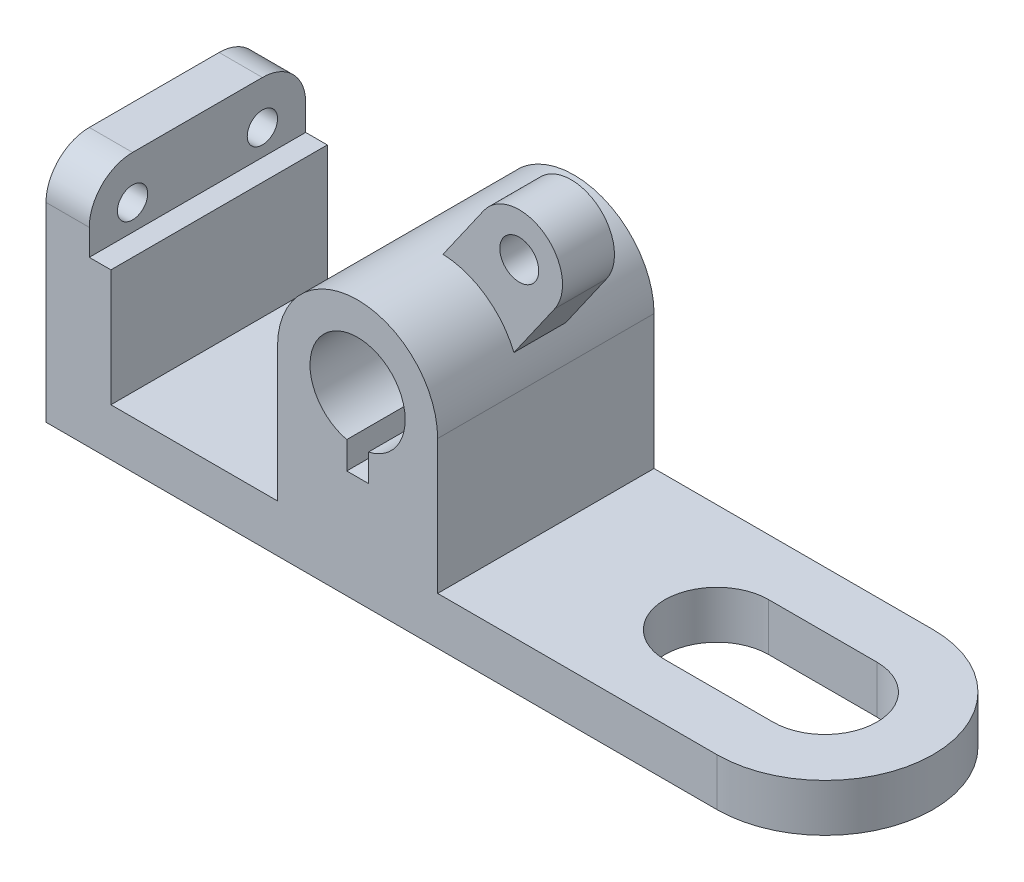
ISO-10303-21;
HEADER;
FILE_DESCRIPTION(('STEP AP214'),'2;1');
FILE_NAME('part.step','',(''),(''),'','','');
FILE_SCHEMA(('AUTOMOTIVE_DESIGN { 1 0 10303 214 1 1 1 1 }'));
ENDSEC;
DATA;
#1=APPLICATION_CONTEXT('core data for automotive mechanical design processes');
#2=APPLICATION_PROTOCOL_DEFINITION('international standard','automotive_design',2000,#1);
#3=PRODUCT_CONTEXT('',#1,'mechanical');
#4=PRODUCT('Part','Part','',(#3));
#5=PRODUCT_RELATED_PRODUCT_CATEGORY('part','',(#4));
#6=PRODUCT_DEFINITION_FORMATION('','',#4);
#7=PRODUCT_DEFINITION_CONTEXT('part definition',#1,'design');
#8=PRODUCT_DEFINITION('design','',#6,#7);
#9=PRODUCT_DEFINITION_SHAPE('','',#8);
#10=(LENGTH_UNIT() NAMED_UNIT(*) SI_UNIT(.MILLI.,.METRE.));
#11=(NAMED_UNIT(*) PLANE_ANGLE_UNIT() SI_UNIT($,.RADIAN.));
#12=(NAMED_UNIT(*) SI_UNIT($,.STERADIAN.) SOLID_ANGLE_UNIT());
#13=UNCERTAINTY_MEASURE_WITH_UNIT(LENGTH_MEASURE(1.E-05),#10,'distance_accuracy_value','');
#14=(GEOMETRIC_REPRESENTATION_CONTEXT(3) GLOBAL_UNCERTAINTY_ASSIGNED_CONTEXT((#13)) GLOBAL_UNIT_ASSIGNED_CONTEXT((#10,
#11,#12)) REPRESENTATION_CONTEXT('',''));
#15=CARTESIAN_POINT('',(0.,0.,0.));
#16=DIRECTION('',(0.,0.,1.));
#17=DIRECTION('',(1.,0.,0.));
#18=AXIS2_PLACEMENT_3D('',#15,#16,#17);
#19=CARTESIAN_POINT('',(0.,38.,0.));
#20=DIRECTION('',(0.,1.,0.));
#21=DIRECTION('',(0.,0.,1.));
#22=AXIS2_PLACEMENT_3D('',#19,#20,#21);
#23=PLANE('',#22);
#24=DIRECTION('',(-1.,0.,0.));
#25=VECTOR('',#24,1.);
#26=CARTESIAN_POINT('',(-62.5,38.,-25.));
#27=LINE('',#26,#25);
#28=CARTESIAN_POINT('',(-62.5,38.,-25.));
#29=VERTEX_POINT('',#28);
#30=CARTESIAN_POINT('',(-67.5,38.,-25.));
#31=VERTEX_POINT('',#30);
#32=EDGE_CURVE('E242',#29,#31,#27,.T.);
#33=ORIENTED_EDGE('',*,*,#32,.T.);
#34=DIRECTION('',(0.,0.,-1.));
#35=VECTOR('',#34,1.);
#36=CARTESIAN_POINT('',(-67.5,38.,25.));
#37=LINE('',#36,#35);
#38=CARTESIAN_POINT('',(-67.5,38.,25.));
#39=VERTEX_POINT('',#38);
#40=EDGE_CURVE('E221',#39,#31,#37,.T.);
#41=ORIENTED_EDGE('',*,*,#40,.F.);
#42=DIRECTION('',(1.,0.,0.));
#43=VECTOR('',#42,1.);
#44=CARTESIAN_POINT('',(-77.5,38.,25.));
#45=LINE('',#44,#43);
#46=CARTESIAN_POINT('',(-62.5,38.,25.));
#47=VERTEX_POINT('',#46);
#48=EDGE_CURVE('E218',#39,#47,#45,.T.);
#49=ORIENTED_EDGE('',*,*,#48,.T.);
#50=DIRECTION('',(0.,0.,-1.));
#51=VECTOR('',#50,1.);
#52=CARTESIAN_POINT('',(-62.5,38.,25.));
#53=LINE('',#52,#51);
#54=EDGE_CURVE('E225',#47,#29,#53,.T.);
#55=ORIENTED_EDGE('',*,*,#54,.T.);
#56=EDGE_LOOP('',(#33,#41,#49,#55));
#57=FACE_BOUND('',#56,.T.);
#58=ADVANCED_FACE('F44',(#57),#23,.T.);
#59=CARTESIAN_POINT('',(77.5,11.,0.));
#60=DIRECTION('',(0.,1.,0.));
#61=DIRECTION('',(0.,0.,1.));
#62=AXIS2_PLACEMENT_3D('',#59,#60,#61);
#63=PLANE('',#62);
#64=DIRECTION('',(-1.,0.,0.));
#65=VECTOR('',#64,1.);
#66=CARTESIAN_POINT('',(-77.5,11.,-25.));
#67=LINE('',#66,#65);
#68=CARTESIAN_POINT('',(-24.,11.,-25.));
#69=VERTEX_POINT('',#68);
#70=CARTESIAN_POINT('',(-62.5,11.,-25.));
#71=VERTEX_POINT('',#70);
#72=EDGE_CURVE('E366',#69,#71,#67,.T.);
#73=ORIENTED_EDGE('',*,*,#72,.T.);
#74=DIRECTION('',(0.,0.,-1.));
#75=VECTOR('',#74,1.);
#76=CARTESIAN_POINT('',(-62.5,11.,25.));
#77=LINE('',#76,#75);
#78=CARTESIAN_POINT('',(-62.5,11.,25.));
#79=VERTEX_POINT('',#78);
#80=EDGE_CURVE('E226',#79,#71,#77,.T.);
#81=ORIENTED_EDGE('',*,*,#80,.F.);
#82=DIRECTION('',(1.,0.,0.));
#83=VECTOR('',#82,1.);
#84=CARTESIAN_POINT('',(77.5,11.,25.));
#85=LINE('',#84,#83);
#86=CARTESIAN_POINT('',(-24.,11.,25.));
#87=VERTEX_POINT('',#86);
#88=EDGE_CURVE('E232',#79,#87,#85,.T.);
#89=ORIENTED_EDGE('',*,*,#88,.T.);
#90=DIRECTION('',(0.,0.,1.));
#91=VECTOR('',#90,1.);
#92=CARTESIAN_POINT('',(-24.,11.,-25.));
#93=LINE('',#92,#91);
#94=EDGE_CURVE('E339',#69,#87,#93,.T.);
#95=ORIENTED_EDGE('',*,*,#94,.F.);
#96=EDGE_LOOP('',(#73,#81,#89,#95));
#97=FACE_BOUND('',#96,.T.);
#98=ADVANCED_FACE('F477',(#97),#63,.T.);
#99=CARTESIAN_POINT('',(52.5,11.,0.));
#100=DIRECTION('',(0.,1.,0.));
#101=DIRECTION('',(0.,0.,1.));
#102=AXIS2_PLACEMENT_3D('',#99,#100,#101);
#103=CIRCLE('',#102,12.);
#104=CARTESIAN_POINT('',(52.5,11.,-12.));
#105=VERTEX_POINT('',#104);
#106=CARTESIAN_POINT('',(52.5,11.,12.));
#107=VERTEX_POINT('',#106);
#108=EDGE_CURVE('E331',#105,#107,#103,.T.);
#109=ORIENTED_EDGE('',*,*,#108,.F.);
#110=DIRECTION('',(-1.,0.,0.));
#111=VECTOR('',#110,1.);
#112=CARTESIAN_POINT('',(52.5,11.,-12.));
#113=LINE('',#112,#111);
#114=CARTESIAN_POINT('',(77.5,11.,-12.));
#115=VERTEX_POINT('',#114);
#116=EDGE_CURVE('E349',#115,#105,#113,.T.);
#117=ORIENTED_EDGE('',*,*,#116,.F.);
#118=CARTESIAN_POINT('',(77.5,11.,0.));
#119=DIRECTION('',(0.,1.,0.));
#120=DIRECTION('',(0.,0.,1.));
#121=AXIS2_PLACEMENT_3D('',#118,#119,#120);
#122=CIRCLE('',#121,12.);
#123=CARTESIAN_POINT('',(77.5,11.,12.));
#124=VERTEX_POINT('',#123);
#125=EDGE_CURVE('E350',#124,#115,#122,.T.);
#126=ORIENTED_EDGE('',*,*,#125,.F.);
#127=DIRECTION('',(1.,0.,0.));
#128=VECTOR('',#127,1.);
#129=CARTESIAN_POINT('',(52.5,11.,12.));
#130=LINE('',#129,#128);
#131=EDGE_CURVE('E341',#107,#124,#130,.T.);
#132=ORIENTED_EDGE('',*,*,#131,.F.);
#133=EDGE_LOOP('',(#109,#117,#126,#132));
#134=FACE_BOUND('',#133,.T.);
#135=CARTESIAN_POINT('',(77.5,11.,-25.));
#136=VERTEX_POINT('',#135);
#137=CARTESIAN_POINT('',(13.,11.,-25.));
#138=VERTEX_POINT('',#137);
#139=EDGE_CURVE('E368',#136,#138,#67,.T.);
#140=ORIENTED_EDGE('',*,*,#139,.T.);
#141=DIRECTION('',(0.,0.,1.));
#142=VECTOR('',#141,1.);
#143=CARTESIAN_POINT('',(13.,11.,-25.));
#144=LINE('',#143,#142);
#145=CARTESIAN_POINT('',(13.,11.,25.));
#146=VERTEX_POINT('',#145);
#147=EDGE_CURVE('E337',#138,#146,#144,.T.);
#148=ORIENTED_EDGE('',*,*,#147,.T.);
#149=CARTESIAN_POINT('',(77.5,11.,25.));
#150=VERTEX_POINT('',#149);
#151=EDGE_CURVE('E371',#146,#150,#85,.T.);
#152=ORIENTED_EDGE('',*,*,#151,.T.);
#153=CARTESIAN_POINT('',(77.5,11.,0.));
#154=DIRECTION('',(0.,1.,0.));
#155=DIRECTION('',(0.,0.,1.));
#156=AXIS2_PLACEMENT_3D('',#153,#154,#155);
#157=CIRCLE('',#156,25.);
#158=EDGE_CURVE('E361',#150,#136,#157,.T.);
#159=ORIENTED_EDGE('',*,*,#158,.T.);
#160=EDGE_LOOP('',(#140,#148,#152,#159));
#161=FACE_BOUND('',#160,.T.);
#162=ADVANCED_FACE('F467',(#134,#161),#63,.T.);
#163=CARTESIAN_POINT('',(77.5,11.,0.));
#164=DIRECTION('',(0.,-1.,0.));
#165=DIRECTION('',(0.,0.,-1.));
#166=AXIS2_PLACEMENT_3D('',#163,#164,#165);
#167=CYLINDRICAL_SURFACE('',#166,25.);
#168=CARTESIAN_POINT('',(77.5,0.,0.));
#169=DIRECTION('',(0.,1.,0.));
#170=DIRECTION('',(0.,0.,1.));
#171=AXIS2_PLACEMENT_3D('',#168,#169,#170);
#172=CIRCLE('',#171,25.);
#173=CARTESIAN_POINT('',(77.5,0.,25.));
#174=VERTEX_POINT('',#173);
#175=CARTESIAN_POINT('',(77.5,0.,-25.));
#176=VERTEX_POINT('',#175);
#177=EDGE_CURVE('E358',#174,#176,#172,.T.);
#178=ORIENTED_EDGE('',*,*,#177,.T.);
#179=DIRECTION('',(0.,-1.,0.));
#180=VECTOR('',#179,1.);
#181=CARTESIAN_POINT('',(77.5,11.,-25.));
#182=LINE('',#181,#180);
#183=EDGE_CURVE('E386',#136,#176,#182,.T.);
#184=ORIENTED_EDGE('',*,*,#183,.F.);
#185=ORIENTED_EDGE('',*,*,#158,.F.);
#186=DIRECTION('',(0.,-1.,0.));
#187=VECTOR('',#186,1.);
#188=CARTESIAN_POINT('',(77.5,11.,25.));
#189=LINE('',#188,#187);
#190=EDGE_CURVE('E373',#150,#174,#189,.T.);
#191=ORIENTED_EDGE('',*,*,#190,.T.);
#192=EDGE_LOOP('',(#178,#184,#185,#191));
#193=FACE_BOUND('',#192,.T.);
#194=ADVANCED_FACE('F457',(#193),#167,.T.);
#195=CARTESIAN_POINT('',(-77.5,11.,-25.));
#196=DIRECTION('',(0.,0.,1.));
#197=DIRECTION('',(1.,0.,0.));
#198=AXIS2_PLACEMENT_3D('',#195,#196,#197);
#199=PLANE('',#198);
#200=CARTESIAN_POINT('',(-5.5,42.,-25.));
#201=DIRECTION('',(0.,0.,1.));
#202=DIRECTION('',(1.,0.,0.));
#203=AXIS2_PLACEMENT_3D('',#200,#201,#202);
#204=CIRCLE('',#203,11.);
#205=CARTESIAN_POINT('',(-3.,31.2878573571857,-25.));
#206=VERTEX_POINT('',#205);
#207=CARTESIAN_POINT('',(-8.,31.2878573571857,-25.));
#208=VERTEX_POINT('',#207);
#209=EDGE_CURVE('E309',#206,#208,#204,.T.);
#210=ORIENTED_EDGE('',*,*,#209,.T.);
#211=DIRECTION('',(0.,-1.,0.));
#212=VECTOR('',#211,1.);
#213=CARTESIAN_POINT('',(-7.99999999999999,11.,-25.));
#214=LINE('',#213,#212);
#215=CARTESIAN_POINT('',(-8.,25.,-25.));
#216=VERTEX_POINT('',#215);
#217=EDGE_CURVE('E312',#208,#216,#214,.T.);
#218=ORIENTED_EDGE('',*,*,#217,.T.);
#219=DIRECTION('',(1.,0.,0.));
#220=VECTOR('',#219,1.);
#221=CARTESIAN_POINT('',(-77.5,25.,-25.));
#222=LINE('',#221,#220);
#223=CARTESIAN_POINT('',(-3.,25.,-25.));
#224=VERTEX_POINT('',#223);
#225=EDGE_CURVE('E299',#216,#224,#222,.T.);
#226=ORIENTED_EDGE('',*,*,#225,.T.);
#227=DIRECTION('',(0.,1.,0.));
#228=VECTOR('',#227,1.);
#229=CARTESIAN_POINT('',(-3.,11.,-25.));
#230=LINE('',#229,#228);
#231=EDGE_CURVE('E310',#224,#206,#230,.T.);
#232=ORIENTED_EDGE('',*,*,#231,.T.);
#233=EDGE_LOOP('',(#210,#218,#226,#232));
#234=FACE_BOUND('',#233,.T.);
#235=DIRECTION('',(0.,-1.,0.));
#236=VECTOR('',#235,1.);
#237=CARTESIAN_POINT('',(-77.5,11.,-25.));
#238=LINE('',#237,#236);
#239=CARTESIAN_POINT('',(-77.5,44.,-25.));
#240=VERTEX_POINT('',#239);
#241=CARTESIAN_POINT('',(-77.5,0.,-25.));
#242=VERTEX_POINT('',#241);
#243=EDGE_CURVE('E390',#240,#242,#238,.T.);
#244=ORIENTED_EDGE('',*,*,#243,.F.);
#245=DIRECTION('',(-1.,0.,0.));
#246=VECTOR('',#245,1.);
#247=CARTESIAN_POINT('',(-67.5,44.,-25.));
#248=LINE('',#247,#246);
#249=CARTESIAN_POINT('',(-67.5,44.,-25.));
#250=VERTEX_POINT('',#249);
#251=EDGE_CURVE('E53',#240,#250,#248,.F.);
#252=ORIENTED_EDGE('',*,*,#251,.T.);
#253=DIRECTION('',(0.,-1.,0.));
#254=VECTOR('',#253,1.);
#255=CARTESIAN_POINT('',(-67.5,54.,-25.));
#256=LINE('',#255,#254);
#257=EDGE_CURVE('E437',#250,#31,#256,.T.);
#258=ORIENTED_EDGE('',*,*,#257,.T.);
#259=ORIENTED_EDGE('',*,*,#32,.F.);
#260=DIRECTION('',(0.,-1.,0.));
#261=VECTOR('',#260,1.);
#262=CARTESIAN_POINT('',(-62.5,38.,-25.));
#263=LINE('',#262,#261);
#264=EDGE_CURVE('E237',#29,#71,#263,.T.);
#265=ORIENTED_EDGE('',*,*,#264,.T.);
#266=ORIENTED_EDGE('',*,*,#72,.F.);
#267=DIRECTION('',(0.,-1.,0.));
#268=VECTOR('',#267,1.);
#269=CARTESIAN_POINT('',(-24.,11.,-25.));
#270=LINE('',#269,#268);
#271=CARTESIAN_POINT('',(-24.,42.,-25.));
#272=VERTEX_POINT('',#271);
#273=EDGE_CURVE('E318',#272,#69,#270,.T.);
#274=ORIENTED_EDGE('',*,*,#273,.F.);
#275=CARTESIAN_POINT('',(-5.5,42.,-25.));
#276=DIRECTION('',(0.,0.,1.));
#277=DIRECTION('',(1.,0.,0.));
#278=AXIS2_PLACEMENT_3D('',#275,#276,#277);
#279=CIRCLE('',#278,18.5);
#280=CARTESIAN_POINT('',(13.,42.,-25.));
#281=VERTEX_POINT('',#280);
#282=EDGE_CURVE('E320',#281,#272,#279,.T.);
#283=ORIENTED_EDGE('',*,*,#282,.F.);
#284=DIRECTION('',(0.,1.,0.));
#285=VECTOR('',#284,1.);
#286=CARTESIAN_POINT('',(13.,42.,-25.));
#287=LINE('',#286,#285);
#288=EDGE_CURVE('E324',#138,#281,#287,.T.);
#289=ORIENTED_EDGE('',*,*,#288,.F.);
#290=ORIENTED_EDGE('',*,*,#139,.F.);
#291=ORIENTED_EDGE('',*,*,#183,.T.);
#292=DIRECTION('',(-1.,0.,0.));
#293=VECTOR('',#292,1.);
#294=CARTESIAN_POINT('',(-77.5,0.,-25.));
#295=LINE('',#294,#293);
#296=EDGE_CURVE('E376',#176,#242,#295,.T.);
#297=ORIENTED_EDGE('',*,*,#296,.T.);
#298=EDGE_LOOP('',(#244,#252,#258,#259,#265,#266,#274,#283,#289,#290,#291,#297));
#299=FACE_BOUND('',#298,.T.);
#300=ADVANCED_FACE('F465',(#234,#299),#199,.F.);
#301=CARTESIAN_POINT('',(-77.5,11.,25.));
#302=DIRECTION('',(1.,0.,0.));
#303=DIRECTION('',(0.,0.,-1.));
#304=AXIS2_PLACEMENT_3D('',#301,#302,#303);
#305=PLANE('',#304);
#306=CARTESIAN_POINT('',(-77.5,44.,15.));
#307=DIRECTION('',(-1.,0.,0.));
#308=DIRECTION('',(0.,0.,1.));
#309=AXIS2_PLACEMENT_3D('',#306,#307,#308);
#310=CIRCLE('',#309,3.5);
#311=CARTESIAN_POINT('',(-77.5,44.,18.5));
#312=VERTEX_POINT('',#311);
#313=EDGE_CURVE('E422',#312,#312,#310,.T.);
#314=ORIENTED_EDGE('',*,*,#313,.F.);
#315=EDGE_LOOP('',(#314));
#316=FACE_BOUND('',#315,.T.);
#317=CARTESIAN_POINT('',(-77.5,44.,-15.));
#318=DIRECTION('',(-1.,0.,0.));
#319=DIRECTION('',(0.,0.,1.));
#320=AXIS2_PLACEMENT_3D('',#317,#318,#319);
#321=CIRCLE('',#320,3.5);
#322=CARTESIAN_POINT('',(-77.5,44.,-11.5));
#323=VERTEX_POINT('',#322);
#324=EDGE_CURVE('E430',#323,#323,#321,.T.);
#325=ORIENTED_EDGE('',*,*,#324,.F.);
#326=EDGE_LOOP('',(#325));
#327=FACE_BOUND('',#326,.T.);
#328=DIRECTION('',(0.,0.,1.));
#329=VECTOR('',#328,1.);
#330=CARTESIAN_POINT('',(-77.5,54.,-25.));
#331=LINE('',#330,#329);
#332=CARTESIAN_POINT('',(-77.5,54.,-15.));
#333=VERTEX_POINT('',#332);
#334=CARTESIAN_POINT('',(-77.5,54.,15.));
#335=VERTEX_POINT('',#334);
#336=EDGE_CURVE('E432',#333,#335,#331,.T.);
#337=ORIENTED_EDGE('',*,*,#336,.F.);
#338=CARTESIAN_POINT('',(-77.5,44.,-15.));
#339=DIRECTION('',(1.,0.,0.));
#340=DIRECTION('',(0.,0.,-1.));
#341=AXIS2_PLACEMENT_3D('',#338,#339,#340);
#342=CIRCLE('',#341,10.);
#343=EDGE_CURVE('E67',#333,#240,#342,.F.);
#344=ORIENTED_EDGE('',*,*,#343,.T.);
#345=ORIENTED_EDGE('',*,*,#243,.T.);
#346=DIRECTION('',(0.,0.,1.));
#347=VECTOR('',#346,1.);
#348=CARTESIAN_POINT('',(-77.5,0.,25.));
#349=LINE('',#348,#347);
#350=CARTESIAN_POINT('',(-77.5,0.,25.));
#351=VERTEX_POINT('',#350);
#352=EDGE_CURVE('E378',#242,#351,#349,.T.);
#353=ORIENTED_EDGE('',*,*,#352,.T.);
#354=DIRECTION('',(0.,-1.,0.));
#355=VECTOR('',#354,1.);
#356=CARTESIAN_POINT('',(-77.5,11.,25.));
#357=LINE('',#356,#355);
#358=CARTESIAN_POINT('',(-77.5,44.,25.));
#359=VERTEX_POINT('',#358);
#360=EDGE_CURVE('E383',#359,#351,#357,.T.);
#361=ORIENTED_EDGE('',*,*,#360,.F.);
#362=CARTESIAN_POINT('',(-77.5,44.,15.));
#363=DIRECTION('',(1.,0.,0.));
#364=DIRECTION('',(0.,0.,-1.));
#365=AXIS2_PLACEMENT_3D('',#362,#363,#364);
#366=CIRCLE('',#365,10.);
#367=EDGE_CURVE('E413',#359,#335,#366,.F.);
#368=ORIENTED_EDGE('',*,*,#367,.T.);
#369=EDGE_LOOP('',(#337,#344,#345,#353,#361,#368));
#370=FACE_BOUND('',#369,.T.);
#371=ADVANCED_FACE('F448',(#316,#327,#370),#305,.F.);
#372=CARTESIAN_POINT('',(77.5,11.,25.));
#373=DIRECTION('',(0.,0.,-1.));
#374=DIRECTION('',(-1.,0.,0.));
#375=AXIS2_PLACEMENT_3D('',#372,#373,#374);
#376=PLANE('',#375);
#377=DIRECTION('',(1.,0.,0.));
#378=VECTOR('',#377,1.);
#379=CARTESIAN_POINT('',(-5.5,25.,25.));
#380=LINE('',#379,#378);
#381=CARTESIAN_POINT('',(-7.99999999999999,25.,25.));
#382=VERTEX_POINT('',#381);
#383=CARTESIAN_POINT('',(-3.,25.,25.));
#384=VERTEX_POINT('',#383);
#385=EDGE_CURVE('E282',#382,#384,#380,.T.);
#386=ORIENTED_EDGE('',*,*,#385,.F.);
#387=DIRECTION('',(0.,-1.,0.));
#388=VECTOR('',#387,1.);
#389=CARTESIAN_POINT('',(-8.,25.,25.));
#390=LINE('',#389,#388);
#391=CARTESIAN_POINT('',(-8.,31.2878573571857,25.));
#392=VERTEX_POINT('',#391);
#393=EDGE_CURVE('E291',#392,#382,#390,.T.);
#394=ORIENTED_EDGE('',*,*,#393,.F.);
#395=CARTESIAN_POINT('',(-5.5,42.,25.));
#396=DIRECTION('',(0.,0.,1.));
#397=DIRECTION('',(1.,0.,0.));
#398=AXIS2_PLACEMENT_3D('',#395,#396,#397);
#399=CIRCLE('',#398,11.);
#400=CARTESIAN_POINT('',(-3.,31.2878573571857,25.));
#401=VERTEX_POINT('',#400);
#402=EDGE_CURVE('E286',#401,#392,#399,.T.);
#403=ORIENTED_EDGE('',*,*,#402,.F.);
#404=DIRECTION('',(0.,1.,0.));
#405=VECTOR('',#404,1.);
#406=CARTESIAN_POINT('',(-3.,25.,25.));
#407=LINE('',#406,#405);
#408=EDGE_CURVE('E290',#384,#401,#407,.T.);
#409=ORIENTED_EDGE('',*,*,#408,.F.);
#410=EDGE_LOOP('',(#386,#394,#403,#409));
#411=FACE_BOUND('',#410,.T.);
#412=DIRECTION('',(0.,-1.,0.));
#413=VECTOR('',#412,1.);
#414=CARTESIAN_POINT('',(-67.5,54.,25.));
#415=LINE('',#414,#413);
#416=CARTESIAN_POINT('',(-67.5,44.,25.));
#417=VERTEX_POINT('',#416);
#418=EDGE_CURVE('E249',#417,#39,#415,.T.);
#419=ORIENTED_EDGE('',*,*,#418,.F.);
#420=DIRECTION('',(1.,0.,0.));
#421=VECTOR('',#420,1.);
#422=CARTESIAN_POINT('',(-77.5,44.,25.));
#423=LINE('',#422,#421);
#424=EDGE_CURVE('E411',#417,#359,#423,.F.);
#425=ORIENTED_EDGE('',*,*,#424,.T.);
#426=ORIENTED_EDGE('',*,*,#360,.T.);
#427=DIRECTION('',(1.,0.,0.));
#428=VECTOR('',#427,1.);
#429=CARTESIAN_POINT('',(77.5,0.,25.));
#430=LINE('',#429,#428);
#431=EDGE_CURVE('E370',#351,#174,#430,.T.);
#432=ORIENTED_EDGE('',*,*,#431,.T.);
#433=ORIENTED_EDGE('',*,*,#190,.F.);
#434=ORIENTED_EDGE('',*,*,#151,.F.);
#435=DIRECTION('',(0.,1.,0.));
#436=VECTOR('',#435,1.);
#437=CARTESIAN_POINT('',(13.,42.,25.));
#438=LINE('',#437,#436);
#439=CARTESIAN_POINT('',(13.,42.,25.));
#440=VERTEX_POINT('',#439);
#441=EDGE_CURVE('E322',#146,#440,#438,.T.);
#442=ORIENTED_EDGE('',*,*,#441,.T.);
#443=CARTESIAN_POINT('',(-5.5,42.,25.));
#444=DIRECTION('',(0.,0.,1.));
#445=DIRECTION('',(1.,0.,0.));
#446=AXIS2_PLACEMENT_3D('',#443,#444,#445);
#447=CIRCLE('',#446,18.5);
#448=CARTESIAN_POINT('',(-24.,42.,25.));
#449=VERTEX_POINT('',#448);
#450=EDGE_CURVE('E317',#440,#449,#447,.T.);
#451=ORIENTED_EDGE('',*,*,#450,.T.);
#452=DIRECTION('',(0.,-1.,0.));
#453=VECTOR('',#452,1.);
#454=CARTESIAN_POINT('',(-24.,11.,25.));
#455=LINE('',#454,#453);
#456=EDGE_CURVE('E327',#449,#87,#455,.T.);
#457=ORIENTED_EDGE('',*,*,#456,.T.);
#458=ORIENTED_EDGE('',*,*,#88,.F.);
#459=DIRECTION('',(0.,-1.,0.));
#460=VECTOR('',#459,1.);
#461=CARTESIAN_POINT('',(-62.5,38.,25.));
#462=LINE('',#461,#460);
#463=EDGE_CURVE('E235',#47,#79,#462,.T.);
#464=ORIENTED_EDGE('',*,*,#463,.F.);
#465=ORIENTED_EDGE('',*,*,#48,.F.);
#466=EDGE_LOOP('',(#419,#425,#426,#432,#433,#434,#442,#451,#457,#458,#464,#465));
#467=FACE_BOUND('',#466,.T.);
#468=ADVANCED_FACE('F231',(#411,#467),#376,.F.);
#469=CARTESIAN_POINT('',(77.5,0.,0.));
#470=DIRECTION('',(0.,1.,0.));
#471=DIRECTION('',(0.,0.,1.));
#472=AXIS2_PLACEMENT_3D('',#469,#470,#471);
#473=PLANE('',#472);
#474=DIRECTION('',(-1.,0.,0.));
#475=VECTOR('',#474,1.);
#476=CARTESIAN_POINT('',(77.5,0.,-12.));
#477=LINE('',#476,#475);
#478=CARTESIAN_POINT('',(77.5,0.,-12.));
#479=VERTEX_POINT('',#478);
#480=CARTESIAN_POINT('',(52.5,0.,-12.));
#481=VERTEX_POINT('',#480);
#482=EDGE_CURVE('E398',#479,#481,#477,.T.);
#483=ORIENTED_EDGE('',*,*,#482,.T.);
#484=CARTESIAN_POINT('',(52.5,0.,0.));
#485=DIRECTION('',(0.,1.,0.));
#486=DIRECTION('',(0.,0.,1.));
#487=AXIS2_PLACEMENT_3D('',#484,#485,#486);
#488=CIRCLE('',#487,12.);
#489=CARTESIAN_POINT('',(52.5,0.,12.));
#490=VERTEX_POINT('',#489);
#491=EDGE_CURVE('E402',#481,#490,#488,.T.);
#492=ORIENTED_EDGE('',*,*,#491,.T.);
#493=DIRECTION('',(1.,0.,0.));
#494=VECTOR('',#493,1.);
#495=CARTESIAN_POINT('',(77.5,0.,12.));
#496=LINE('',#495,#494);
#497=CARTESIAN_POINT('',(77.5,0.,12.));
#498=VERTEX_POINT('',#497);
#499=EDGE_CURVE('E395',#490,#498,#496,.T.);
#500=ORIENTED_EDGE('',*,*,#499,.T.);
#501=CARTESIAN_POINT('',(77.5,0.,0.));
#502=DIRECTION('',(0.,1.,0.));
#503=DIRECTION('',(0.,0.,1.));
#504=AXIS2_PLACEMENT_3D('',#501,#502,#503);
#505=CIRCLE('',#504,12.);
#506=EDGE_CURVE('E394',#498,#479,#505,.T.);
#507=ORIENTED_EDGE('',*,*,#506,.T.);
#508=EDGE_LOOP('',(#483,#492,#500,#507));
#509=FACE_BOUND('',#508,.T.);
#510=ORIENTED_EDGE('',*,*,#177,.F.);
#511=ORIENTED_EDGE('',*,*,#431,.F.);
#512=ORIENTED_EDGE('',*,*,#352,.F.);
#513=ORIENTED_EDGE('',*,*,#296,.F.);
#514=EDGE_LOOP('',(#510,#511,#512,#513));
#515=FACE_BOUND('',#514,.T.);
#516=ADVANCED_FACE('F462',(#509,#515),#473,.F.);
#517=CARTESIAN_POINT('',(52.5,-91.,0.));
#518=DIRECTION('',(0.,1.,0.));
#519=DIRECTION('',(0.,0.,1.));
#520=AXIS2_PLACEMENT_3D('',#517,#518,#519);
#521=CYLINDRICAL_SURFACE('',#520,12.);
#522=DIRECTION('',(0.,1.,0.));
#523=VECTOR('',#522,1.);
#524=CARTESIAN_POINT('',(52.5,-91.,-12.));
#525=LINE('',#524,#523);
#526=EDGE_CURVE('E354',#481,#105,#525,.T.);
#527=ORIENTED_EDGE('',*,*,#526,.T.);
#528=ORIENTED_EDGE('',*,*,#108,.T.);
#529=DIRECTION('',(0.,1.,0.));
#530=VECTOR('',#529,1.);
#531=CARTESIAN_POINT('',(52.5,-91.,12.));
#532=LINE('',#531,#530);
#533=EDGE_CURVE('E353',#490,#107,#532,.T.);
#534=ORIENTED_EDGE('',*,*,#533,.F.);
#535=ORIENTED_EDGE('',*,*,#491,.F.);
#536=EDGE_LOOP('',(#527,#528,#534,#535));
#537=FACE_BOUND('',#536,.T.);
#538=ADVANCED_FACE('F556',(#537),#521,.F.);
#539=CARTESIAN_POINT('',(52.5,-91.,-12.));
#540=DIRECTION('',(0.,0.,-1.));
#541=DIRECTION('',(-1.,0.,0.));
#542=AXIS2_PLACEMENT_3D('',#539,#540,#541);
#543=PLANE('',#542);
#544=DIRECTION('',(0.,1.,0.));
#545=VECTOR('',#544,1.);
#546=CARTESIAN_POINT('',(77.5,-91.,-12.));
#547=LINE('',#546,#545);
#548=EDGE_CURVE('E357',#479,#115,#547,.T.);
#549=ORIENTED_EDGE('',*,*,#548,.T.);
#550=ORIENTED_EDGE('',*,*,#116,.T.);
#551=ORIENTED_EDGE('',*,*,#526,.F.);
#552=ORIENTED_EDGE('',*,*,#482,.F.);
#553=EDGE_LOOP('',(#549,#550,#551,#552));
#554=FACE_BOUND('',#553,.T.);
#555=ADVANCED_FACE('F555',(#554),#543,.F.);
#556=CARTESIAN_POINT('',(77.5,-91.,0.));
#557=DIRECTION('',(0.,1.,0.));
#558=DIRECTION('',(0.,0.,1.));
#559=AXIS2_PLACEMENT_3D('',#556,#557,#558);
#560=CYLINDRICAL_SURFACE('',#559,12.);
#561=DIRECTION('',(0.,1.,0.));
#562=VECTOR('',#561,1.);
#563=CARTESIAN_POINT('',(77.5,-91.,12.));
#564=LINE('',#563,#562);
#565=EDGE_CURVE('E360',#498,#124,#564,.T.);
#566=ORIENTED_EDGE('',*,*,#565,.T.);
#567=ORIENTED_EDGE('',*,*,#125,.T.);
#568=ORIENTED_EDGE('',*,*,#548,.F.);
#569=ORIENTED_EDGE('',*,*,#506,.F.);
#570=EDGE_LOOP('',(#566,#567,#568,#569));
#571=FACE_BOUND('',#570,.T.);
#572=ADVANCED_FACE('F560',(#571),#560,.F.);
#573=CARTESIAN_POINT('',(52.5,-91.,12.));
#574=DIRECTION('',(0.,0.,1.));
#575=DIRECTION('',(1.,0.,0.));
#576=AXIS2_PLACEMENT_3D('',#573,#574,#575);
#577=PLANE('',#576);
#578=ORIENTED_EDGE('',*,*,#533,.T.);
#579=ORIENTED_EDGE('',*,*,#131,.T.);
#580=ORIENTED_EDGE('',*,*,#565,.F.);
#581=ORIENTED_EDGE('',*,*,#499,.F.);
#582=EDGE_LOOP('',(#578,#579,#580,#581));
#583=FACE_BOUND('',#582,.T.);
#584=ADVANCED_FACE('F552',(#583),#577,.F.);
#585=CARTESIAN_POINT('',(-5.5,42.,-25.));
#586=DIRECTION('',(0.,0.,1.));
#587=DIRECTION('',(1.,0.,0.));
#588=AXIS2_PLACEMENT_3D('',#585,#586,#587);
#589=CYLINDRICAL_SURFACE('',#588,18.5);
#590=CARTESIAN_POINT('',(-5.5,42.,6.));
#591=DIRECTION('',(0.,0.,-1.));
#592=DIRECTION('',(1.,0.,0.));
#593=AXIS2_PLACEMENT_3D('',#590,#591,#592);
#594=CIRCLE('',#593,18.5);
#595=CARTESIAN_POINT('',(-4.764157442559,60.4853600378964,6.));
#596=VERTEX_POINT('',#595);
#597=CARTESIAN_POINT('',(11.6188834432209,49.0138313108756,6.));
#598=VERTEX_POINT('',#597);
#599=EDGE_CURVE('E253',#596,#598,#594,.T.);
#600=ORIENTED_EDGE('',*,*,#599,.F.);
#601=DIRECTION('',(0.,0.,-1.));
#602=VECTOR('',#601,1.);
#603=CARTESIAN_POINT('',(-4.764157442559,60.4853600378964,6.));
#604=LINE('',#603,#602);
#605=CARTESIAN_POINT('',(-4.764157442559,60.4853600378964,-6.));
#606=VERTEX_POINT('',#605);
#607=EDGE_CURVE('E264',#596,#606,#604,.T.);
#608=ORIENTED_EDGE('',*,*,#607,.T.);
#609=CARTESIAN_POINT('',(-5.5,42.,-6.));
#610=DIRECTION('',(0.,0.,-1.));
#611=DIRECTION('',(1.,0.,0.));
#612=AXIS2_PLACEMENT_3D('',#609,#610,#611);
#613=CIRCLE('',#612,18.5);
#614=CARTESIAN_POINT('',(11.6188834432209,49.0138313108756,-6.));
#615=VERTEX_POINT('',#614);
#616=EDGE_CURVE('E267',#606,#615,#613,.T.);
#617=ORIENTED_EDGE('',*,*,#616,.T.);
#618=DIRECTION('',(0.,0.,-1.));
#619=VECTOR('',#618,1.);
#620=CARTESIAN_POINT('',(11.6188834432209,49.0138313108756,6.));
#621=LINE('',#620,#619);
#622=EDGE_CURVE('E285',#598,#615,#621,.T.);
#623=ORIENTED_EDGE('',*,*,#622,.F.);
#624=EDGE_LOOP('',(#600,#608,#617,#623));
#625=FACE_BOUND('',#624,.T.);
#626=ORIENTED_EDGE('',*,*,#450,.F.);
#627=DIRECTION('',(0.,0.,1.));
#628=VECTOR('',#627,1.);
#629=CARTESIAN_POINT('',(13.,42.,-25.));
#630=LINE('',#629,#628);
#631=EDGE_CURVE('E333',#281,#440,#630,.T.);
#632=ORIENTED_EDGE('',*,*,#631,.F.);
#633=ORIENTED_EDGE('',*,*,#282,.T.);
#634=DIRECTION('',(0.,0.,1.));
#635=VECTOR('',#634,1.);
#636=CARTESIAN_POINT('',(-24.,42.,-25.));
#637=LINE('',#636,#635);
#638=EDGE_CURVE('E326',#272,#449,#637,.T.);
#639=ORIENTED_EDGE('',*,*,#638,.T.);
#640=EDGE_LOOP('',(#626,#632,#633,#639));
#641=FACE_BOUND('',#640,.T.);
#642=ADVANCED_FACE('F472',(#625,#641),#589,.T.);
#643=CARTESIAN_POINT('',(13.,42.,-25.));
#644=DIRECTION('',(1.,0.,0.));
#645=DIRECTION('',(0.,1.,0.));
#646=AXIS2_PLACEMENT_3D('',#643,#644,#645);
#647=PLANE('',#646);
#648=ORIENTED_EDGE('',*,*,#441,.F.);
#649=ORIENTED_EDGE('',*,*,#147,.F.);
#650=ORIENTED_EDGE('',*,*,#288,.T.);
#651=ORIENTED_EDGE('',*,*,#631,.T.);
#652=EDGE_LOOP('',(#648,#649,#650,#651));
#653=FACE_BOUND('',#652,.T.);
#654=ADVANCED_FACE('F469',(#653),#647,.T.);
#655=CARTESIAN_POINT('',(-24.,11.,-25.));
#656=DIRECTION('',(-1.,0.,0.));
#657=DIRECTION('',(0.,-1.,0.));
#658=AXIS2_PLACEMENT_3D('',#655,#656,#657);
#659=PLANE('',#658);
#660=ORIENTED_EDGE('',*,*,#456,.F.);
#661=ORIENTED_EDGE('',*,*,#638,.F.);
#662=ORIENTED_EDGE('',*,*,#273,.T.);
#663=ORIENTED_EDGE('',*,*,#94,.T.);
#664=EDGE_LOOP('',(#660,#661,#662,#663));
#665=FACE_BOUND('',#664,.T.);
#666=ADVANCED_FACE('F473',(#665),#659,.T.);
#667=CARTESIAN_POINT('',(-8.,25.,-43.));
#668=DIRECTION('',(-1.,0.,0.));
#669=DIRECTION('',(0.,0.,1.));
#670=AXIS2_PLACEMENT_3D('',#667,#668,#669);
#671=PLANE('',#670);
#672=DIRECTION('',(0.,0.,1.));
#673=VECTOR('',#672,1.);
#674=CARTESIAN_POINT('',(-8.,31.2878573571857,-43.));
#675=LINE('',#674,#673);
#676=EDGE_CURVE('E297',#208,#392,#675,.T.);
#677=ORIENTED_EDGE('',*,*,#676,.T.);
#678=ORIENTED_EDGE('',*,*,#393,.T.);
#679=DIRECTION('',(0.,0.,1.));
#680=VECTOR('',#679,1.);
#681=CARTESIAN_POINT('',(-8.,25.,-43.));
#682=LINE('',#681,#680);
#683=EDGE_CURVE('E298',#216,#382,#682,.T.);
#684=ORIENTED_EDGE('',*,*,#683,.F.);
#685=ORIENTED_EDGE('',*,*,#217,.F.);
#686=EDGE_LOOP('',(#677,#678,#684,#685));
#687=FACE_BOUND('',#686,.T.);
#688=ADVANCED_FACE('F532',(#687),#671,.F.);
#689=CARTESIAN_POINT('',(-5.5,42.,-43.));
#690=DIRECTION('',(0.,0.,1.));
#691=DIRECTION('',(1.,0.,0.));
#692=AXIS2_PLACEMENT_3D('',#689,#690,#691);
#693=CYLINDRICAL_SURFACE('',#692,11.);
#694=DIRECTION('',(0.,0.,1.));
#695=VECTOR('',#694,1.);
#696=CARTESIAN_POINT('',(-3.,31.2878573571857,-43.));
#697=LINE('',#696,#695);
#698=EDGE_CURVE('E305',#206,#401,#697,.T.);
#699=ORIENTED_EDGE('',*,*,#698,.T.);
#700=ORIENTED_EDGE('',*,*,#402,.T.);
#701=ORIENTED_EDGE('',*,*,#676,.F.);
#702=ORIENTED_EDGE('',*,*,#209,.F.);
#703=EDGE_LOOP('',(#699,#700,#701,#702));
#704=FACE_BOUND('',#703,.T.);
#705=ADVANCED_FACE('F534',(#704),#693,.F.);
#706=CARTESIAN_POINT('',(-3.,25.,-43.));
#707=DIRECTION('',(1.,0.,0.));
#708=DIRECTION('',(0.,0.,-1.));
#709=AXIS2_PLACEMENT_3D('',#706,#707,#708);
#710=PLANE('',#709);
#711=DIRECTION('',(0.,0.,1.));
#712=VECTOR('',#711,1.);
#713=CARTESIAN_POINT('',(-3.,25.,-43.));
#714=LINE('',#713,#712);
#715=EDGE_CURVE('E294',#224,#384,#714,.T.);
#716=ORIENTED_EDGE('',*,*,#715,.T.);
#717=ORIENTED_EDGE('',*,*,#408,.T.);
#718=ORIENTED_EDGE('',*,*,#698,.F.);
#719=ORIENTED_EDGE('',*,*,#231,.F.);
#720=EDGE_LOOP('',(#716,#717,#718,#719));
#721=FACE_BOUND('',#720,.T.);
#722=ADVANCED_FACE('F539',(#721),#710,.F.);
#723=CARTESIAN_POINT('',(-5.5,25.,-43.));
#724=DIRECTION('',(0.,-1.,0.));
#725=DIRECTION('',(0.,0.,-1.));
#726=AXIS2_PLACEMENT_3D('',#723,#724,#725);
#727=PLANE('',#726);
#728=ORIENTED_EDGE('',*,*,#683,.T.);
#729=ORIENTED_EDGE('',*,*,#385,.T.);
#730=ORIENTED_EDGE('',*,*,#715,.F.);
#731=ORIENTED_EDGE('',*,*,#225,.F.);
#732=EDGE_LOOP('',(#728,#729,#730,#731));
#733=FACE_BOUND('',#732,.T.);
#734=ADVANCED_FACE('F529',(#733),#727,.F.);
#735=CARTESIAN_POINT('',(11.6188834432209,49.0138313108756,6.));
#736=DIRECTION('',(-0.819152044288993,0.573576436351044,0.));
#737=DIRECTION('',(-0.573576436351044,-0.819152044288994,0.));
#738=AXIS2_PLACEMENT_3D('',#735,#736,#737);
#739=PLANE('',#738);
#740=DIRECTION('',(0.573576436351044,0.819152044288993,0.));
#741=VECTOR('',#740,1.);
#742=CARTESIAN_POINT('',(11.6188834432209,49.0138313108756,-6.));
#743=LINE('',#742,#741);
#744=CARTESIAN_POINT('',(21.0459664061233,62.4771010537374,-6.));
#745=VERTEX_POINT('',#744);
#746=EDGE_CURVE('E269',#615,#745,#743,.T.);
#747=ORIENTED_EDGE('',*,*,#746,.T.);
#748=DIRECTION('',(0.,0.,-1.));
#749=VECTOR('',#748,1.);
#750=CARTESIAN_POINT('',(21.0459664061233,62.4771010537374,6.));
#751=LINE('',#750,#749);
#752=CARTESIAN_POINT('',(21.0459664061233,62.4771010537374,6.));
#753=VERTEX_POINT('',#752);
#754=EDGE_CURVE('E276',#753,#745,#751,.T.);
#755=ORIENTED_EDGE('',*,*,#754,.F.);
#756=DIRECTION('',(0.573576436351044,0.819152044288993,0.));
#757=VECTOR('',#756,1.);
#758=CARTESIAN_POINT('',(11.6188834432209,49.0138313108756,6.));
#759=LINE('',#758,#757);
#760=EDGE_CURVE('E259',#598,#753,#759,.T.);
#761=ORIENTED_EDGE('',*,*,#760,.F.);
#762=ORIENTED_EDGE('',*,*,#622,.T.);
#763=EDGE_LOOP('',(#747,#755,#761,#762));
#764=FACE_BOUND('',#763,.T.);
#765=ADVANCED_FACE('F524',(#764),#739,.F.);
#766=CARTESIAN_POINT('',(12.8544459632334,68.2128654172478,6.));
#767=DIRECTION('',(0.,0.,-1.));
#768=DIRECTION('',(-1.,0.,0.));
#769=AXIS2_PLACEMENT_3D('',#766,#767,#768);
#770=CYLINDRICAL_SURFACE('',#769,10.);
#771=CARTESIAN_POINT('',(12.8544459632334,68.2128654172478,-6.));
#772=DIRECTION('',(0.,0.,1.));
#773=DIRECTION('',(1.,0.,0.));
#774=AXIS2_PLACEMENT_3D('',#771,#772,#773);
#775=CIRCLE('',#774,10.);
#776=CARTESIAN_POINT('',(4.66292552034348,73.9486297807583,-6.));
#777=VERTEX_POINT('',#776);
#778=EDGE_CURVE('E272',#745,#777,#775,.T.);
#779=ORIENTED_EDGE('',*,*,#778,.T.);
#780=DIRECTION('',(0.,0.,-1.));
#781=VECTOR('',#780,1.);
#782=CARTESIAN_POINT('',(4.66292552034348,73.9486297807583,6.));
#783=LINE('',#782,#781);
#784=CARTESIAN_POINT('',(4.66292552034348,73.9486297807583,6.));
#785=VERTEX_POINT('',#784);
#786=EDGE_CURVE('E277',#785,#777,#783,.T.);
#787=ORIENTED_EDGE('',*,*,#786,.F.);
#788=CARTESIAN_POINT('',(12.8544459632334,68.2128654172478,6.));
#789=DIRECTION('',(0.,0.,1.));
#790=DIRECTION('',(1.,0.,0.));
#791=AXIS2_PLACEMENT_3D('',#788,#789,#790);
#792=CIRCLE('',#791,10.);
#793=EDGE_CURVE('E261',#753,#785,#792,.T.);
#794=ORIENTED_EDGE('',*,*,#793,.F.);
#795=ORIENTED_EDGE('',*,*,#754,.T.);
#796=EDGE_LOOP('',(#779,#787,#794,#795));
#797=FACE_BOUND('',#796,.T.);
#798=ADVANCED_FACE('F521',(#797),#770,.T.);
#799=CARTESIAN_POINT('',(-4.764157442559,60.4853600378964,6.));
#800=DIRECTION('',(0.819152044288993,-0.573576436351044,0.));
#801=DIRECTION('',(0.573576436351044,0.819152044288993,0.));
#802=AXIS2_PLACEMENT_3D('',#799,#800,#801);
#803=PLANE('',#802);
#804=DIRECTION('',(-0.573576436351044,-0.819152044288993,0.));
#805=VECTOR('',#804,1.);
#806=CARTESIAN_POINT('',(-4.764157442559,60.4853600378964,-6.));
#807=LINE('',#806,#805);
#808=EDGE_CURVE('E256',#777,#606,#807,.T.);
#809=ORIENTED_EDGE('',*,*,#808,.T.);
#810=ORIENTED_EDGE('',*,*,#607,.F.);
#811=DIRECTION('',(-0.573576436351044,-0.819152044288993,0.));
#812=VECTOR('',#811,1.);
#813=CARTESIAN_POINT('',(-4.764157442559,60.4853600378964,6.));
#814=LINE('',#813,#812);
#815=EDGE_CURVE('E263',#785,#596,#814,.T.);
#816=ORIENTED_EDGE('',*,*,#815,.F.);
#817=ORIENTED_EDGE('',*,*,#786,.T.);
#818=EDGE_LOOP('',(#809,#810,#816,#817));
#819=FACE_BOUND('',#818,.T.);
#820=ADVANCED_FACE('F511',(#819),#803,.F.);
#821=CARTESIAN_POINT('',(-5.5,42.,6.));
#822=DIRECTION('',(0.,0.,1.));
#823=DIRECTION('',(1.,0.,0.));
#824=AXIS2_PLACEMENT_3D('',#821,#822,#823);
#825=PLANE('',#824);
#826=CARTESIAN_POINT('',(12.8544459632334,68.2128654172478,6.));
#827=DIRECTION('',(0.,0.,1.));
#828=DIRECTION('',(1.,0.,0.));
#829=AXIS2_PLACEMENT_3D('',#826,#827,#828);
#830=CIRCLE('',#829,4.5);
#831=CARTESIAN_POINT('',(17.3544459632334,68.2128654172478,6.));
#832=VERTEX_POINT('',#831);
#833=EDGE_CURVE('E238',#832,#832,#830,.T.);
#834=ORIENTED_EDGE('',*,*,#833,.F.);
#835=EDGE_LOOP('',(#834));
#836=FACE_BOUND('',#835,.T.);
#837=ORIENTED_EDGE('',*,*,#599,.T.);
#838=ORIENTED_EDGE('',*,*,#760,.T.);
#839=ORIENTED_EDGE('',*,*,#793,.T.);
#840=ORIENTED_EDGE('',*,*,#815,.T.);
#841=EDGE_LOOP('',(#837,#838,#839,#840));
#842=FACE_BOUND('',#841,.T.);
#843=ADVANCED_FACE('F512',(#836,#842),#825,.T.);
#844=CARTESIAN_POINT('',(-5.5,42.,-6.));
#845=DIRECTION('',(0.,0.,1.));
#846=DIRECTION('',(1.,0.,0.));
#847=AXIS2_PLACEMENT_3D('',#844,#845,#846);
#848=PLANE('',#847);
#849=CARTESIAN_POINT('',(12.8544459632334,68.2128654172478,-6.));
#850=DIRECTION('',(0.,0.,1.));
#851=DIRECTION('',(1.,0.,0.));
#852=AXIS2_PLACEMENT_3D('',#849,#850,#851);
#853=CIRCLE('',#852,4.5);
#854=CARTESIAN_POINT('',(17.3544459632334,68.2128654172478,-6.));
#855=VERTEX_POINT('',#854);
#856=EDGE_CURVE('E251',#855,#855,#853,.T.);
#857=ORIENTED_EDGE('',*,*,#856,.T.);
#858=EDGE_LOOP('',(#857));
#859=FACE_BOUND('',#858,.T.);
#860=ORIENTED_EDGE('',*,*,#616,.F.);
#861=ORIENTED_EDGE('',*,*,#808,.F.);
#862=ORIENTED_EDGE('',*,*,#778,.F.);
#863=ORIENTED_EDGE('',*,*,#746,.F.);
#864=EDGE_LOOP('',(#860,#861,#862,#863));
#865=FACE_BOUND('',#864,.T.);
#866=ADVANCED_FACE('F508',(#859,#865),#848,.F.);
#867=CARTESIAN_POINT('',(12.8544459632334,68.2128654172478,-14.));
#868=DIRECTION('',(0.,0.,1.));
#869=DIRECTION('',(1.,0.,0.));
#870=AXIS2_PLACEMENT_3D('',#867,#868,#869);
#871=CYLINDRICAL_SURFACE('',#870,4.5);
#872=ORIENTED_EDGE('',*,*,#833,.T.);
#873=EDGE_LOOP('',(#872));
#874=FACE_BOUND('',#873,.T.);
#875=ORIENTED_EDGE('',*,*,#856,.F.);
#876=EDGE_LOOP('',(#875));
#877=FACE_BOUND('',#876,.T.);
#878=ADVANCED_FACE('F506',(#874,#877),#871,.F.);
#879=CARTESIAN_POINT('',(-62.5,38.,25.));
#880=DIRECTION('',(-1.,0.,0.));
#881=DIRECTION('',(0.,0.,1.));
#882=AXIS2_PLACEMENT_3D('',#879,#880,#881);
#883=PLANE('',#882);
#884=ORIENTED_EDGE('',*,*,#80,.T.);
#885=ORIENTED_EDGE('',*,*,#264,.F.);
#886=ORIENTED_EDGE('',*,*,#54,.F.);
#887=ORIENTED_EDGE('',*,*,#463,.T.);
#888=EDGE_LOOP('',(#884,#885,#886,#887));
#889=FACE_BOUND('',#888,.T.);
#890=ADVANCED_FACE('F241',(#889),#883,.F.);
#891=CARTESIAN_POINT('',(-67.5,54.,25.));
#892=DIRECTION('',(-1.,0.,0.));
#893=DIRECTION('',(0.,0.,1.));
#894=AXIS2_PLACEMENT_3D('',#891,#892,#893);
#895=PLANE('',#894);
#896=CARTESIAN_POINT('',(-67.5,44.,15.));
#897=DIRECTION('',(-1.,0.,0.));
#898=DIRECTION('',(0.,0.,1.));
#899=AXIS2_PLACEMENT_3D('',#896,#897,#898);
#900=CIRCLE('',#899,3.5);
#901=CARTESIAN_POINT('',(-67.5,44.,18.5));
#902=VERTEX_POINT('',#901);
#903=EDGE_CURVE('E47',#902,#902,#900,.T.);
#904=ORIENTED_EDGE('',*,*,#903,.T.);
#905=EDGE_LOOP('',(#904));
#906=FACE_BOUND('',#905,.T.);
#907=CARTESIAN_POINT('',(-67.5,44.,-15.));
#908=DIRECTION('',(-1.,0.,0.));
#909=DIRECTION('',(0.,0.,1.));
#910=AXIS2_PLACEMENT_3D('',#907,#908,#909);
#911=CIRCLE('',#910,3.5);
#912=CARTESIAN_POINT('',(-67.5,44.,-11.5));
#913=VERTEX_POINT('',#912);
#914=EDGE_CURVE('E416',#913,#913,#911,.T.);
#915=ORIENTED_EDGE('',*,*,#914,.T.);
#916=EDGE_LOOP('',(#915));
#917=FACE_BOUND('',#916,.T.);
#918=ORIENTED_EDGE('',*,*,#257,.F.);
#919=CARTESIAN_POINT('',(-67.5,44.,-15.));
#920=DIRECTION('',(-1.,0.,0.));
#921=DIRECTION('',(0.,0.,1.));
#922=AXIS2_PLACEMENT_3D('',#919,#920,#921);
#923=CIRCLE('',#922,10.);
#924=CARTESIAN_POINT('',(-67.5,54.,-15.));
#925=VERTEX_POINT('',#924);
#926=EDGE_CURVE('E11',#250,#925,#923,.F.);
#927=ORIENTED_EDGE('',*,*,#926,.T.);
#928=DIRECTION('',(0.,0.,-1.));
#929=VECTOR('',#928,1.);
#930=CARTESIAN_POINT('',(-67.5,54.,25.));
#931=LINE('',#930,#929);
#932=CARTESIAN_POINT('',(-67.5,54.,15.));
#933=VERTEX_POINT('',#932);
#934=EDGE_CURVE('E436',#933,#925,#931,.T.);
#935=ORIENTED_EDGE('',*,*,#934,.F.);
#936=CARTESIAN_POINT('',(-67.5,44.,15.));
#937=DIRECTION('',(-1.,0.,0.));
#938=DIRECTION('',(0.,0.,1.));
#939=AXIS2_PLACEMENT_3D('',#936,#937,#938);
#940=CIRCLE('',#939,10.);
#941=EDGE_CURVE('E406',#933,#417,#940,.F.);
#942=ORIENTED_EDGE('',*,*,#941,.T.);
#943=ORIENTED_EDGE('',*,*,#418,.T.);
#944=ORIENTED_EDGE('',*,*,#40,.T.);
#945=EDGE_LOOP('',(#918,#927,#935,#942,#943,#944));
#946=FACE_BOUND('',#945,.T.);
#947=ADVANCED_FACE('F445',(#906,#917,#946),#895,.F.);
#948=CARTESIAN_POINT('',(0.,54.,0.));
#949=DIRECTION('',(0.,1.,0.));
#950=DIRECTION('',(0.,0.,1.));
#951=AXIS2_PLACEMENT_3D('',#948,#949,#950);
#952=PLANE('',#951);
#953=ORIENTED_EDGE('',*,*,#934,.T.);
#954=DIRECTION('',(-1.,0.,0.));
#955=VECTOR('',#954,1.);
#956=CARTESIAN_POINT('',(-77.5,54.,-15.));
#957=LINE('',#956,#955);
#958=EDGE_CURVE('E417',#925,#333,#957,.T.);
#959=ORIENTED_EDGE('',*,*,#958,.T.);
#960=ORIENTED_EDGE('',*,*,#336,.T.);
#961=DIRECTION('',(1.,0.,0.));
#962=VECTOR('',#961,1.);
#963=CARTESIAN_POINT('',(-67.5,54.,15.));
#964=LINE('',#963,#962);
#965=EDGE_CURVE('E404',#335,#933,#964,.T.);
#966=ORIENTED_EDGE('',*,*,#965,.T.);
#967=EDGE_LOOP('',(#953,#959,#960,#966));
#968=FACE_BOUND('',#967,.T.);
#969=ADVANCED_FACE('F484',(#968),#952,.T.);
#970=CARTESIAN_POINT('',(0.,44.,15.));
#971=DIRECTION('',(-1.,0.,0.));
#972=DIRECTION('',(0.,0.,1.));
#973=AXIS2_PLACEMENT_3D('',#970,#971,#972);
#974=CYLINDRICAL_SURFACE('',#973,10.);
#975=ORIENTED_EDGE('',*,*,#367,.F.);
#976=ORIENTED_EDGE('',*,*,#424,.F.);
#977=ORIENTED_EDGE('',*,*,#941,.F.);
#978=ORIENTED_EDGE('',*,*,#965,.F.);
#979=EDGE_LOOP('',(#975,#976,#977,#978));
#980=FACE_BOUND('',#979,.T.);
#981=ADVANCED_FACE('F449',(#980),#974,.T.);
#982=CARTESIAN_POINT('',(0.,44.,-15.));
#983=DIRECTION('',(1.,0.,0.));
#984=DIRECTION('',(0.,0.,-1.));
#985=AXIS2_PLACEMENT_3D('',#982,#983,#984);
#986=CYLINDRICAL_SURFACE('',#985,10.);
#987=ORIENTED_EDGE('',*,*,#926,.F.);
#988=ORIENTED_EDGE('',*,*,#251,.F.);
#989=ORIENTED_EDGE('',*,*,#343,.F.);
#990=ORIENTED_EDGE('',*,*,#958,.F.);
#991=EDGE_LOOP('',(#987,#988,#989,#990));
#992=FACE_BOUND('',#991,.T.);
#993=ADVANCED_FACE('F50',(#992),#986,.T.);
#994=CARTESIAN_POINT('',(-61.5,44.,-15.));
#995=DIRECTION('',(-1.,0.,0.));
#996=DIRECTION('',(0.,0.,1.));
#997=AXIS2_PLACEMENT_3D('',#994,#995,#996);
#998=CYLINDRICAL_SURFACE('',#997,3.5);
#999=ORIENTED_EDGE('',*,*,#324,.T.);
#1000=EDGE_LOOP('',(#999));
#1001=FACE_BOUND('',#1000,.T.);
#1002=ORIENTED_EDGE('',*,*,#914,.F.);
#1003=EDGE_LOOP('',(#1002));
#1004=FACE_BOUND('',#1003,.T.);
#1005=ADVANCED_FACE('F750',(#1001,#1004),#998,.F.);
#1006=CARTESIAN_POINT('',(-61.5,44.,15.));
#1007=DIRECTION('',(-1.,0.,0.));
#1008=DIRECTION('',(0.,0.,1.));
#1009=AXIS2_PLACEMENT_3D('',#1006,#1007,#1008);
#1010=CYLINDRICAL_SURFACE('',#1009,3.5);
#1011=ORIENTED_EDGE('',*,*,#313,.T.);
#1012=EDGE_LOOP('',(#1011));
#1013=FACE_BOUND('',#1012,.T.);
#1014=ORIENTED_EDGE('',*,*,#903,.F.);
#1015=EDGE_LOOP('',(#1014));
#1016=FACE_BOUND('',#1015,.T.);
#1017=ADVANCED_FACE('F760',(#1013,#1016),#1010,.F.);
#1018=CLOSED_SHELL('',(#58,#98,#162,#194,#300,#371,#468,#516,#538,#555,#572,#584,#642,#654,#666,
#688,#705,#722,#734,#765,#798,#820,#843,#866,#878,#890,#947,#969,#981,#993,#1005,#1017));
#1019=MANIFOLD_SOLID_BREP('B2',#1018);
#1020=ADVANCED_BREP_SHAPE_REPRESENTATION('',(#18,#1019),#14);
#1021=SHAPE_DEFINITION_REPRESENTATION(#9,#1020);
ENDSEC;
END-ISO-10303-21;
